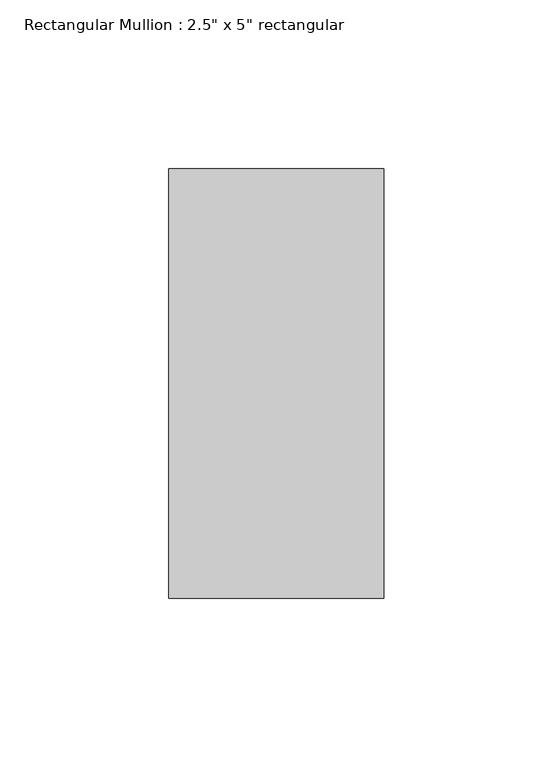
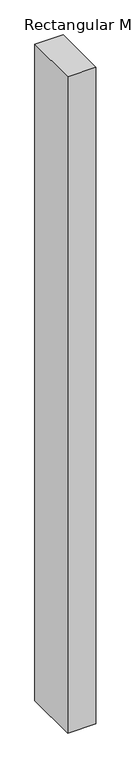
"""IFC4 building model written with IfcOpenShell, lengths in millimetres: member geometry."""

from ifc_helpers import new_model, si_unit, frame, origin, place, context, project, spatial, polyline, outline, extrude, source, transform, mapped, element, save


def member_3a7ae77e(model_context):
    return source(origin(), model_context, "Body", "SweptSolid", [
        extrude(outline(polyline([(31.75, 63.5), (31.75, -63.5), (-31.75, -63.5), (-31.75, 63.5), (31.75, 63.5)])), frame((0.0, 0.0, -1556.4785779), z_axis=(0.0, 0.0, 1.0), x_axis=(1.0, 0.0, 0.0)), (0.0, 0.0, 1.0), 1556.4785779),
    ])


if __name__ == "__main__":
    model = new_model("IFC4")
    model_context = context("Model", 3, world=origin())
    ifc_project = project(units=[si_unit("LENGTHUNIT", "METRE", prefix="MILLI")], contexts=[model_context])
    site = spatial("IfcSite", under=ifc_project)
    building = spatial("IfcBuilding", under=site)
    placement = place(None, origin())
    member_shape = member_3a7ae77e(model_context)
    element("IfcMember", 1, ObjectType="Rectangular Mullion : 2.5\" x 5\" rectangular", at=placement, inside=building, context=model_context, shape_type="MappedRepresentation", body=[
        mapped(member_shape, transform((0.0, 0.0, 0.0), x_axis=(1.0, 0.0, 0.0), y_axis=(0.0, 1.0, 0.0), z_axis=(0.0, 0.0, 1.0))),
    ])
    save(model, "model.ifc")

# Revit data of these elements
# Type "Rectangular Mullion : 2.5\" x 5\" rectangular"
#   built-in parameter 1007304 = 0.416667 (stored number, unit not read)
#   built-in parameter 1007301 = 0.104167 (stored number, unit not read)
#   built-in parameter 1007300 = 0.104167 (stored number, unit not read)
# Element 1 (IfcMember, "Rectangular Mullion : 2.5\" x 5\" rectangular")
#   Materials on its faces: "Aluminum"
# Materials
#   "Aluminum": class "Metal", colour RGB 247 247 247, transparency 0, Description = "Aluminum 6061", Cost = 0
